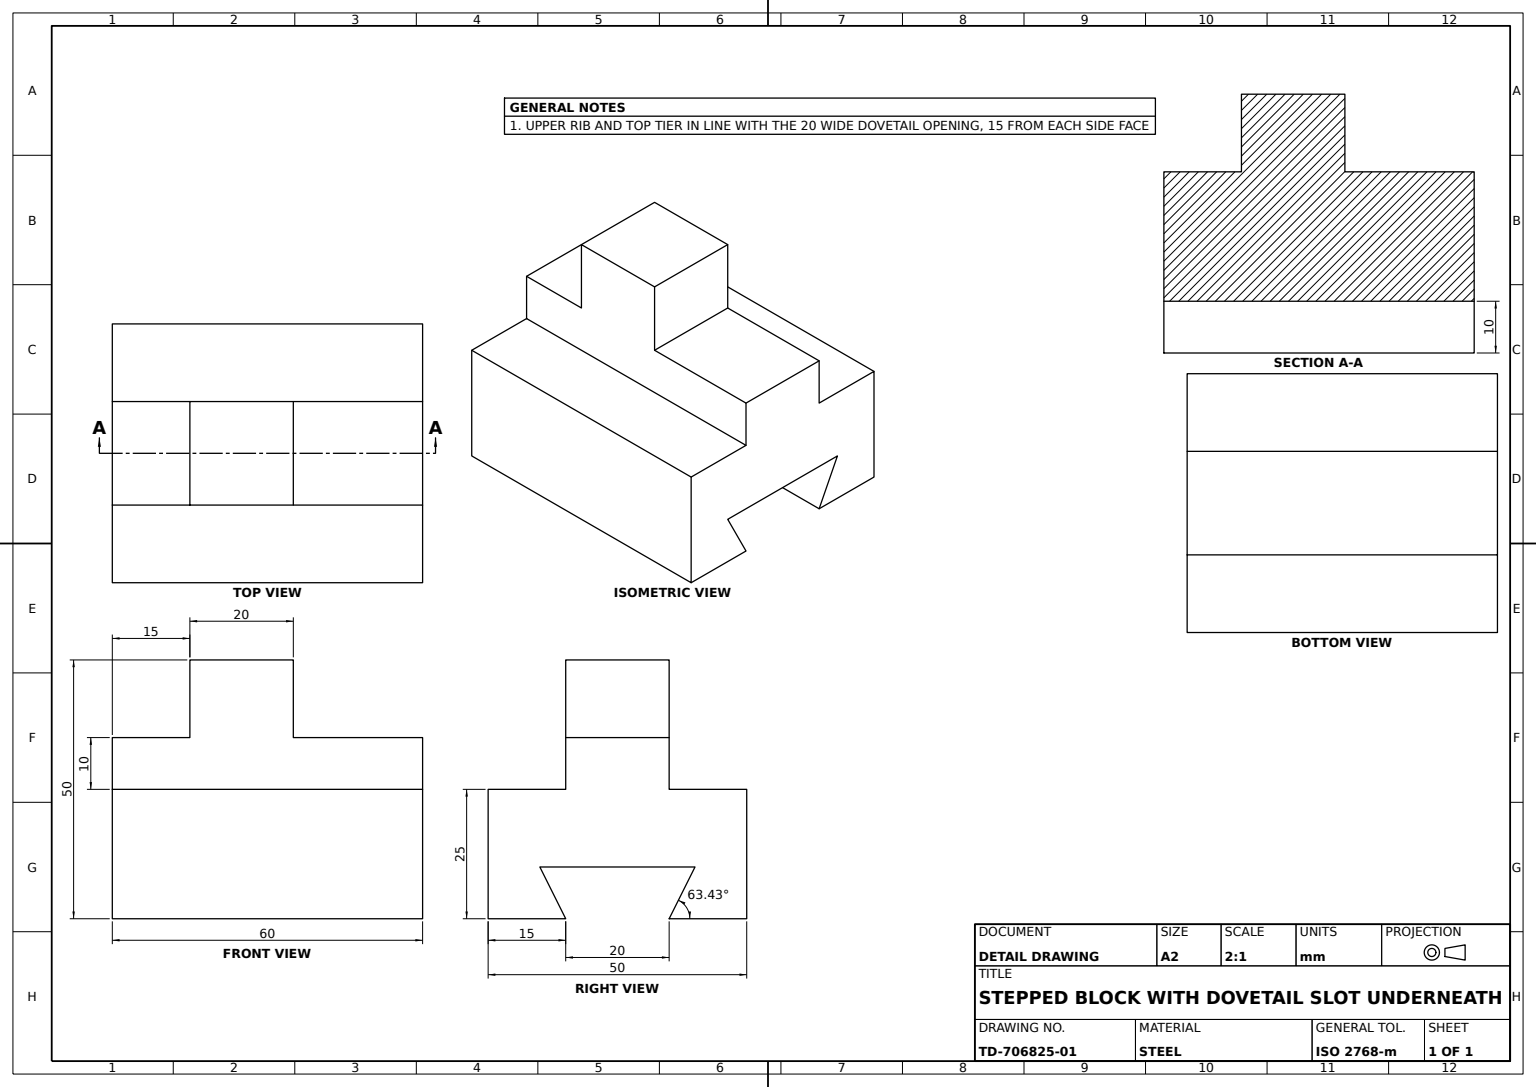
SolidWorks part; units mm, degrees
material "Plain Carbon Steel"
ref_plane "Front Plane" through (0, 0, 0) normal (0, 0, 1) x (1, 0, 0)
ref_plane "Top Plane" through (0, 0, 0) normal (0, 1, 0) x (1, 0, 0)
ref_plane "Right Plane" through (0, 0, 0) normal (1, 0, 0) x (0, 0, -1)
sketch "Stepped Block Profile Sketch" plane through (0, 0, 0) normal (1, 0, 0) x (0, 0, -1)
  line L0 (-25, 0) -> (25, 0)
  line L1 (25, 0) -> (25, 25)
  line L2 (25, 25) -> (10, 25)
  line L3 (10, 25) -> (10, 50)
  line L4 (10, 50) -> (-10, 50)
  line L5 (-10, 50) -> (-10, 25)
  line L6 (-10, 25) -> (-25, 25)
  line L7 (-25, 25) -> (-25, 0)
  point P7 (0, 50)
  dimension "D1" = 50
  dimension "D2" = 20
  dimension "D3" = 25
  dimension "D4" = 25
extrude "Stepped Block 60mm" add sketch "Stepped Block Profile Sketch" along normal mid plane 60
sketch "Underside Dovetail Groove Sketch" plane through (0, 0, 10) normal (0, 0, 1) x (1, 0, 0)
  line L0 (-30, 25) -> (-30, 35)
  line L1 (-30, 50) -> (-30, 25) construction
  line L2 (-30, 35) -> (-15, 35)
  line L3 (-15, 35) -> (-15, 50)
  line L4 (30, 50) -> (-30, 50) construction
  line L5 (-15, 50) -> (5, 50)
  line L6 (5, 50) -> (5, 35)
  line L7 (5, 35) -> (30, 35)
  line L8 (30, 50) -> (30, 25) construction
  line L9 (30, 35) -> (30, 25)
  line L10 (30, 25) -> (-30, 25)
  line M9 (-30, 50) -> (-30, 25)
  line M11 (30, 25) -> (30, 50)
  line M12 (30, 50) -> (-30, 50)
  dimension "D1" = 20
  dimension "D2" = 15
  dimension "D3" = 15
extrude "Underside Dovetail Groove" cut sketch "Underside Dovetail Groove Sketch" against normal up to next contours L2 L3 M12 M9 | L6 L7 M11 M12
sketch "Top Tier Pocket Sketch" plane through (30, 0, 0) normal (1, 0, 0) x (0, 0, -1)
  line L0 (-10, 0) -> (-15, 10)
  line L1 (-25, 0) -> (25, 0) construction
  line L2 (-15, 10) -> (15, 10)
  line L3 (15, 10) -> (10, 0)
  line L4 (10, 0) -> (-10, 0)
  point P4 (0, 10)
  point P9 (0, 0)
  dimension "D1" = 30
  dimension "D2" = 20
  dimension "D3" = 10
extrude "Top Tier Pocket 30x20" cut sketch "Top Tier Pocket Sketch" against normal up to next
